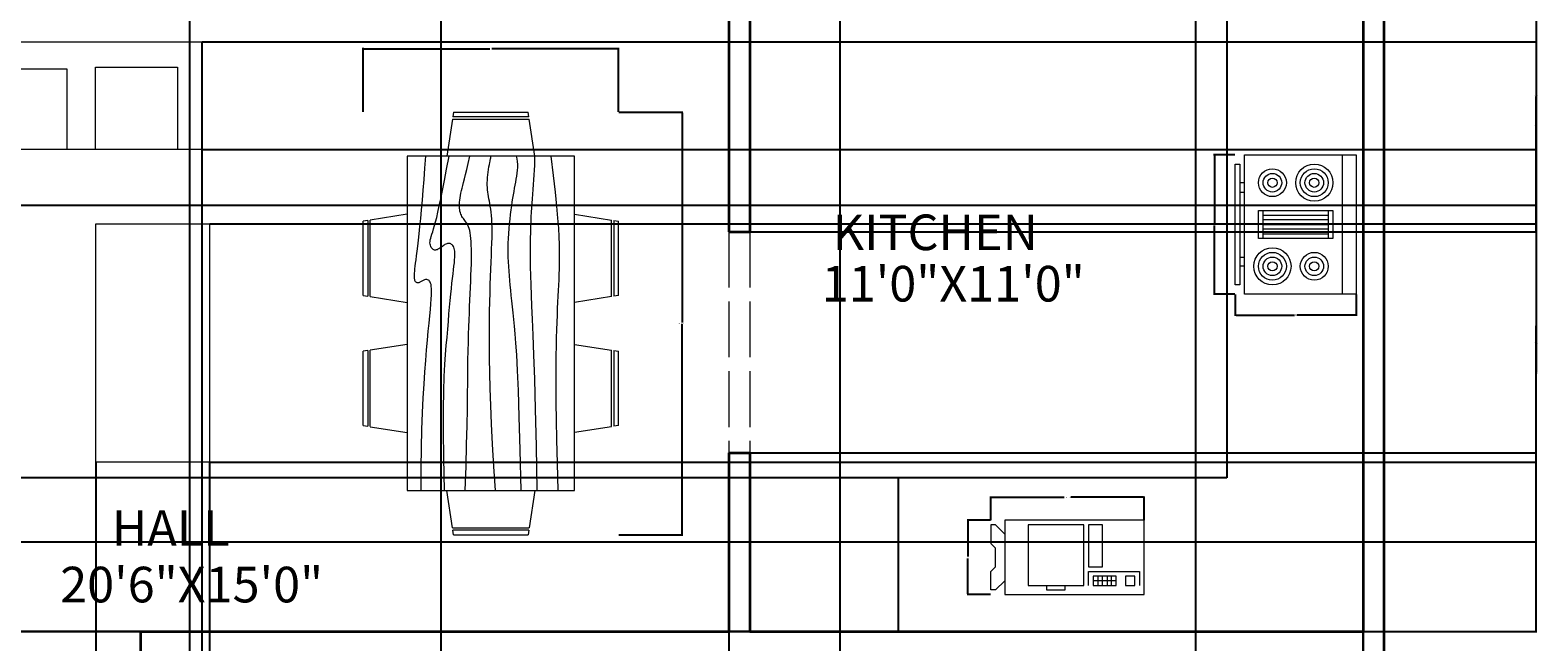
# Model space of a CAD drawing. Units: inches. Extents: x 2337 to 2851, y 1463 to 2183.
# Tile 3 of 4: x 2527 to 2851, y 1810 to 1942. Entities that reach past the tile are written whole.
import ezdxf

# ---------------------------------------------------------------- set-up
doc = ezdxf.new("R2010")
doc.units = ezdxf.units.IN
doc.linetypes.add('ACAD_ISO02W100', pattern=[15, 12, -3])
for name, color, linetype, lineweight in [('A-ANNO-DIMS', 2, 'Continuous', 18), ('A-AREA-IDEN', 7, 'Continuous', 18), ('A-EQPM', 9, 'Continuous', 18), ('A-FLOR-CASE', 8, 'Continuous', 25), ('A-FURN', 8, 'Continuous', 18), ('A-WALL', 7, 'Continuous', 35), ('A-WALL-OVHD', 7, 'ACAD_ISO02W100', 18)]:
    doc.layers.add(name, color=color, linetype=linetype, lineweight=lineweight)
doc.styles.get("Standard").update_dxf_attribs({"font": 'arial.ttf'})
doc.dimstyles.get("Standard").update_dxf_attribs({"dimtxt": 0.18, "dimasz": 0.18, "dimexe": 0.18, "dimexo": 0.0625, "dimgap": 0.09, "dimtad": 0, "dimtih": 1, "dimtoh": 1, "dimdec": 4, "dimzin": 0, "dimdsep": 46, "dimtxsty": 'Standard', "dimcen": 0.09, "dimadec": 0, "dimazin": 0, "dimtfac": 1, "dimtdec": 4, "dimtofl": 0, "dimtmove": 0, "dimatfit": 3, "dimfxl": 1, "dimtolj": 1, "dimtzin": 0, "dimarcsym": 0})

# ---------------------------------------------------------------- blocks, each defined once
blk = doc.blocks.new('Range-Oven - 30 in top')
for p, q in [((0, -3), (30, -3)), ((12, -6), (18, -6)), ((13, -20), (13, -6)), ((14, -6), (14, -20)), ((15, -20), (15, -6)), ((16, -6), (16, -20)), ((17, -20), (17, -6)), ((18, -20), (12, -20)), ((6, -24), (6, -25)), ((8, -25), (8, -24)), ((22, -25), (22, -24)), ((24, -24), (24, -25))]:
    blk.add_line(p, q)
for points in [[(0, -24), (0, 0), (30, 0), (30, -24)], [(12, -21), (12, -5), (18, -5), (18, -21)], [(2, -26), (2, -25), (28, -25), (28, -26)]]:
    blk.add_lwpolyline(points, close=True)
for centre, radius in [((6, -9), 4), ((6, -9), 3), ((24, -9), 3), ((6, -9), 2), ((6, -9), 1), ((24, -9), 2), ((24, -9), 1), ((6, -18), 3), ((6, -18), 2), ((24, -18), 4), ((24, -18), 3), ((24, -18), 2), ((6, -18), 1), ((24, -18), 1)]:
    blk.add_circle(centre, radius)
blk = doc.blocks.new('Copy Machine')
for p, q in [((0, 0), (0, -16)), ((30, 0), (0, 0)), ((30, -16), (30, 0)), ((-3, -1), (-3, -5)), ((-2, -1), (-3, -1)), ((0, -3), (-2, -1)), ((5, -1), (5, -14)), ((17, -1), (5, -1)), ((17, -14), (17, -1)), ((18, -1), (18, -10)), ((21, -1), (18, -1)), ((21, -10), (21, -1)), ((-3, -5), (-2, -6)), ((-2, -10), (-2, -6)), ((-3, -11), (-2, -10)), ((-3, -15), (-3, -11)), ((18, -10), (21, -10)), ((18, -14), (18, -11)), ((18, -11), (29, -11)), ((24, -12), (19, -12)), ((19, -12), (19, -14)), ((20, -12), (20, -14)), ((21, -14), (21, -12)), ((22, -12), (22, -14)), ((23, -14), (23, -12)), ((24, -14), (24, -12)), ((28, -12), (26, -12)), ((26, -12), (26, -14)), ((28, -14), (28, -12)), ((29, -11), (29, -14)), ((-2, -15), (-3, -15)), ((0, -13), (-2, -15)), ((0, -16), (30, -16)), ((5, -14), (17, -14)), ((9, -14), (9, -15)), ((9, -15), (13, -15)), ((13, -15), (13, -14)), ((24, -13), (19, -13)), ((19, -14), (24, -14)), ((26, -14), (28, -14))]:
    blk.add_line(p, q)
blk = doc.blocks.new('Dining Set - 36 x 72 in.')
for p, q in [((-22.2343, 26.00059), (-23.4847, 17.99762)), ((-22.2304, 26), (-5.7608, 26)), ((-22, 27.5), (-22.1562, 26.50042)), ((-5.8416, 26.5), (-22.1534, 26.5)), ((-22, 27.5), (-6, 27.5)), ((-5.8437, 26.49966), (-6, 27.5)), ((-4.5152, 17.99762), (-5.7655, 25.99926)), ((5.7657, 26.00059), (4.5153, 17.99762)), ((5.7696, 26), (22.2392, 26)), ((6, 27.5), (5.8438, 26.50042)), ((22.1584, 26.5), (5.8466, 26.5)), ((6, 27.5), (22, 27.5)), ((22.1563, 26.49966), (22, 27.5)), ((23.4848, 17.99762), (22.2345, 25.99926)), ((36, 18), (-36, 18)), ((-36, 18), (-36, -18)), ((36, -18), (36, 18)), ((-45.5, 8), (-44.5004, 8.15617)), ((-45.5, 8), (-45.5, -8)), ((-44.5, -8.15843), (-44.5, 8.15338)), ((-44.0006, 8.23428), (-35.9976, 9.48474)), ((-44, 8.23041), (-44, -8.23915)), ((44.0006, 8.23428), (35.9976, 9.48474)), ((44, 8.23041), (44, -8.23915)), ((44.5, -8.15843), (44.5, 8.15338)), ((45.5, 8), (44.5005, 8.15617)), ((45.5, 8), (45.5, -8)), ((-44.4997, -8.15631), (-45.5, -8)), ((-35.9976, -9.48476), (-43.9993, -8.2345)), ((35.9976, -9.48476), (43.9993, -8.2345)), ((44.4997, -8.15631), (45.5, -8)), ((-36, -18), (36, -18)), ((-22.2343, -26.0006), (-23.4847, -17.99762)), ((-4.5152, -17.99762), (-5.7655, -25.99928)), ((5.7657, -26.0006), (4.5153, -17.99762)), ((23.4848, -17.99762), (22.2345, -25.99928)), ((-22.2304, -26), (-5.7608, -26)), ((-22, -27.5), (-22.1562, -26.50044)), ((-5.8416, -26.5), (-22.1534, -26.5)), ((-22, -27.5), (-6, -27.5)), ((-5.8437, -26.49967), (-6, -27.5)), ((5.7696, -26), (22.2392, -26)), ((6, -27.5), (5.8438, -26.50044)), ((22.1584, -26.5), (5.8466, -26.5)), ((6, -27.5), (22, -27.5)), ((22.1563, -26.49967), (22, -27.5))]:
    blk.add_line(p, q)
for points in [[(-36, 15), (-31.1772, 14.97754), (-26.8079, 14.91406), (-22.8538, 14.81543), (-19.276, 14.6875), (-16.0362, 14.53613), (-13.0957, 14.36718), (-10.4159, 14.18652), (-7.9583, 14), (-5.6904, 13.81315), (-3.6035, 13.63021), (-1.6954, 13.45508), (0.0365, 13.29166), (1.5945, 13.14388), (2.9811, 13.01562), (4.1988, 12.9108), (5.25, 12.83333), (6.1393, 12.78613), (6.8802, 12.76823), (7.4883, 12.77767), (7.9792, 12.8125), (8.3685, 12.87077), (8.6719, 12.95052), (8.9049, 13.0498), (9.0833, 13.16666), (9.2205, 13.29899), (9.3216, 13.44401), (9.3895, 13.59879), (9.4271, 13.76041), (9.4373, 13.92594), (9.4232, 14.09245), (9.3875, 14.257), (9.3333, 14.41666), (9.2638, 14.56917), (9.1836, 14.71484), (9.0975, 14.85465), (9.0104, 14.98958), (8.9272, 15.1206), (8.8529, 15.2487), (8.7922, 15.37483), (8.75, 15.5), (8.7305, 15.62467), (8.7344, 15.74739), (8.7617, 15.86621), (8.8125, 15.97916), (8.8867, 16.08431), (8.9844, 16.17968), (9.1055, 16.26334), (9.25, 16.33333), (9.4189, 16.38802), (9.6172, 16.42708), (9.8506, 16.45052), (10.125, 16.45833), (10.4463, 16.45052), (10.8203, 16.42708), (11.2529, 16.38802), (11.75, 16.33333), (12.3184, 16.26318), (12.9694, 16.17838), (13.7151, 16.07991), (14.5677, 15.96875), (15.5395, 15.84586), (16.6426, 15.71224), (17.8893, 15.56884), (19.2917, 15.41666), (20.859, 15.25667), (22.5879, 15.08984), (24.4721, 14.91715), (26.5052, 14.73958), (28.6809, 14.5581), (30.9929, 14.3737), (33.4347, 14.18733), (36, 14)], [(-36, 10), (-28.9766, 10.14274), (-23.1725, 10.20442), (-18.4241, 10.19775), (-14.5677, 10.13541), (-11.4399, 10.03011), (-8.877, 9.89453), (-6.7154, 9.74137), (-4.7917, 9.58333), (-2.9698, 9.43082), (-1.2246, 9.28515), (0.4415, 9.14534), (2.026, 9.01041), (3.5266, 8.87939), (4.9408, 8.7513), (6.266, 8.62516), (7.5, 8.5), (8.6411, 8.37549), (9.6914, 8.2539), (10.6538, 8.13818), (11.5312, 8.03125), (12.3267, 7.93603), (13.043, 7.85547), (13.6831, 7.79248), (14.25, 7.75), (14.7471, 7.7303), (15.1797, 7.73307), (15.5537, 7.75732), (15.875, 7.80208), (16.1494, 7.86637), (16.3828, 7.94922), (16.5811, 8.04964), (16.75, 8.16666), (16.8944, 8.29915), (17.0143, 8.44531), (17.1089, 8.60319), (17.1771, 8.77083), (17.218, 8.94629), (17.2305, 9.1276), (17.2137, 9.31282), (17.1667, 9.5), (17.0895, 9.6875), (16.987, 9.875), (16.8649, 10.0625), (16.7292, 10.25), (16.5856, 10.4375), (16.4401, 10.625), (16.2985, 10.8125), (16.1667, 11), (16.05, 11.18733), (15.9518, 11.3737), (15.8752, 11.5581), (15.8229, 11.73958), (15.798, 11.91715), (15.8034, 12.08984), (15.842, 12.25667), (15.9167, 12.41666), (16.0295, 12.56836), (16.1784, 12.70833), (16.3605, 12.83268), (16.5729, 12.9375), (16.8127, 13.01888), (17.0768, 13.07291), (17.3625, 13.0957), (17.6667, 13.08333), (17.9894, 13.03312), (18.3418, 12.94726), (18.7382, 12.82918), (19.1927, 12.68229), (19.7195, 12.51001), (20.3327, 12.31575), (21.0465, 12.10294), (21.875, 11.875), (22.8357, 11.63354), (23.959, 11.37304), (25.2786, 11.08618), (26.8282, 10.76562), (28.6414, 10.40405), (30.752, 9.99414), (33.1936, 9.52856), (36, 9)], [(-36, 5.5), (-30.7157, 5.3348), (-26.069, 5.20963), (-21.9946, 5.11767), (-18.4271, 5.05208), (-15.3009, 5.00602), (-12.5508, 4.97265), (-10.1112, 4.94515), (-7.9167, 4.91666), (-5.909, 4.88167), (-4.0586, 4.83984), (-2.3429, 4.79215), (-0.7396, 4.73958), (0.7739, 4.6831), (2.22, 4.6237), (3.6213, 4.56233), (5, 4.5), (6.373, 4.43782), (7.7344, 4.3776), (9.0723, 4.32129), (10.375, 4.27083), (11.6309, 4.22819), (12.8281, 4.19531), (13.9551, 4.17415), (15, 4.16666), (15.954, 4.17448), (16.819, 4.19791), (17.6001, 4.23698), (18.3021, 4.29166), (18.9299, 4.36198), (19.4883, 4.44791), (19.9823, 4.54948), (20.4167, 4.66666), (20.7969, 4.79899), (21.1302, 4.94401), (21.4245, 5.09879), (21.6875, 5.26041), (21.9271, 5.42594), (22.1511, 5.59245), (22.3672, 5.757), (22.5834, 5.91666), (22.8065, 6.06868), (23.0404, 6.21093), (23.2879, 6.34147), (23.5521, 6.45833), (23.8358, 6.55957), (24.142, 6.64323), (24.4735, 6.70735), (24.8334, 6.75), (25.2235, 6.76969), (25.642, 6.76692), (26.0858, 6.74267), (26.5521, 6.69791), (27.0379, 6.63362), (27.5404, 6.55078), (28.0565, 6.45036), (28.5834, 6.33333), (29.1242, 6.19987), (29.7071, 6.04687), (30.3661, 5.87044), (31.1354, 5.66666), (32.0493, 5.43164), (33.142, 5.16146), (34.4475, 4.85221), (36, 4.5)], [(-36, -1), (-30.7915, -0.6591), (-26.0195, -0.38216), (-21.6519, -0.16284), (-17.6563, 0.00521), (-14.0005, 0.12833), (-10.6523, 0.21289), (-7.5796, 0.26522), (-4.75, 0.29166), (-2.134, 0.29793), (0.2878, 0.28711), (2.5317, 0.26163), (4.6146, 0.22396), (6.5529, 0.17651), (8.3633, 0.12174), (10.0623, 0.06209), (11.6667, 0), (13.1899, -0.06201), (14.6341, -0.1211), (15.9982, -0.17432), (17.2813, -0.21875), (18.4823, -0.25147), (19.6003, -0.26953), (20.6343, -0.27002), (21.5834, -0.25), (22.4481, -0.20768), (23.2357, -0.14584), (23.9549, -0.06836), (24.6146, 0.02083), (25.2235, 0.11784), (25.7904, 0.21875), (26.3241, 0.31966), (26.8334, 0.41666), (27.3265, 0.50618), (27.8099, 0.58593), (28.2894, 0.65397), (28.7709, 0.70833), (29.2601, 0.74707), (29.763, 0.76823), (30.2855, 0.76985), (30.8334, 0.75), (31.4088, 0.70784), (31.9994, 0.64713), (32.589, 0.57275), (33.1615, 0.48958), (33.7008, 0.4025), (34.1908, 0.3164), (34.6153, 0.23616), (34.9584, 0.16666), (35.2099, 0.11165), (35.3848, 0.07031), (35.504, 0.04069), (35.5886, 0.02083), (35.6594, 0.00879), (35.7377, 0.0026), (35.8442, 0.00032), (36, 0)], [(-36, -6.5), (-27.1843, -6.31267), (-20.084, -6.1263), (-14.469, -5.9419), (-10.1094, -5.76042), (-6.7752, -5.58285), (-4.2363, -5.41016), (-2.2629, -5.24333), (-0.625, -5.08334), (0.8708, -4.93099), (2.2715, -4.78646), (3.5872, -4.64974), (4.8281, -4.52084), (6.0046, -4.39974), (7.127, -4.28646), (8.2053, -4.18099), (9.25, -4.08334), (10.2705, -3.99382), (11.2734, -3.91407), (12.2647, -3.84603), (13.25, -3.79167), (14.2354, -3.75293), (15.2266, -3.73177), (16.2295, -3.73015), (17.25, -3.75), (18.2912, -3.79248), (19.3451, -3.85547), (20.4009, -3.93604), (21.4479, -4.03125), (22.4754, -4.13819), (23.4727, -4.25391), (24.4289, -4.37549), (25.3334, -4.5), (26.1785, -4.62492), (26.9694, -4.74935), (27.7145, -4.87281), (28.4219, -4.99479), (29.1, -5.11483), (29.7572, -5.23242), (30.4016, -5.34709), (31.0417, -5.45834), (31.6837, -5.56437), (32.3262, -5.65821), (32.9658, -5.73153), (33.599, -5.77604), (34.2224, -5.78345), (34.8327, -5.74545), (35.4264, -5.65373), (36, -5.5)], [(-36, -10), (-26.4022, -9.81299), (-18.4675, -9.62891), (-11.9839, -9.45069), (-6.7396, -9.28125), (-2.5226, -9.12354), (0.8789, -8.98047), (3.6769, -8.85498), (6.0833, -8.75), (8.2767, -8.66765), (10.3021, -8.60677), (12.1712, -8.56543), (13.8958, -8.54167), (15.4876, -8.53353), (16.9583, -8.53907), (18.3197, -8.55632), (19.5834, -8.58334), (20.7616, -8.61841), (21.8685, -8.66081), (22.9188, -8.71004), (23.9271, -8.76563), (24.9081, -8.82707), (25.8763, -8.89388), (26.8465, -8.96558), (27.8334, -9.04167), (28.8474, -9.12118), (29.8828, -9.20117), (30.93, -9.27824), (31.9792, -9.34896), (33.0205, -9.40991), (34.0443, -9.45768), (35.0407, -9.48885), (36, -9.5)], [(-36, -14.5), (-30.0881, -14.33513), (-25.0332, -14.21224), (-20.7312, -14.12647), (-17.0781, -14.07292), (-13.97, -14.04671), (-11.3027, -14.04297), (-8.9724, -14.05681), (-6.875, -14.08334), (-4.9224, -14.11833), (-3.0905, -14.16016), (-1.3709, -14.20785), (0.2448, -14.26042), (1.7647, -14.3169), (3.1973, -14.3763), (4.5507, -14.43767), (5.8333, -14.5), (7.0554, -14.5621), (8.235, -14.62175), (9.3922, -14.67652), (10.5469, -14.72396), (11.7192, -14.76164), (12.929, -14.78711), (14.1965, -14.79794), (15.5417, -14.79167), (16.9933, -14.76424), (18.6152, -14.70508), (20.4804, -14.60197), (22.6615, -14.44271), (25.2312, -14.21509), (28.2624, -13.9069), (31.8277, -13.50594), (36, -13)]]:
    blk.add_lwpolyline(points)
blk = doc.blocks.new('*D23')
at = {"layer": 'A-ANNO-DIMS', "color": 0, "lineweight": -2, "transparency": 16777216}
for p, q in [((2785.97, 1914.93), (2781.36, 1914.93)), ((2781.54, 1914.75), (2781.54, 1900.11)), ((2781.54, 1885.11), (2781.54, 1899.75)), ((2785.97, 1884.93), (2781.36, 1884.93))]:
    blk.add_line(p, q, dxfattribs=at)
at = {"layer": 'A-ANNO-DIMS', "color": 0, "transparency": 16777216}
for points in [[(2781.51, 1914.75), (2781.57, 1914.75), (2781.54, 1914.93)], [(2781.51, 1885.11), (2781.57, 1885.11), (2781.54, 1884.93)]]:
    blk.add_solid(points, dxfattribs=at)
at = {"layer": 'Defpoints', "color": 0, "transparency": 16777216}
for p in [(2786.04, 1914.93), (2781.54, 1884.93), (2786.04, 1884.93)]:
    blk.add_point(p, dxfattribs=at)
at = {"layer": 'A-ANNO-DIMS', "color": 0, "transparency": 16777216, "insert": (2781.54, 1899.93), "char_height": 0.18, "attachment_point": 5}
blk.add_mtext('\\A1;RANGE 30', dxfattribs=at)
blk = doc.blocks.new('*D24')
at = {"layer": 'A-ANNO-DIMS', "color": 0, "lineweight": -2, "transparency": 16777216}
for p, q in [((2786.04, 1884.87), (2786.04, 1880.25)), ((2812.04, 1884.87), (2812.04, 1880.25)), ((2786.22, 1880.43), (2798.81, 1880.43)), ((2811.86, 1880.43), (2799.26, 1880.43))]:
    blk.add_line(p, q, dxfattribs=at)
at = {"layer": 'A-ANNO-DIMS', "color": 0, "transparency": 16777216}
for points in [[(2786.22, 1880.46), (2786.22, 1880.4), (2786.04, 1880.43)], [(2811.86, 1880.46), (2811.86, 1880.4), (2812.04, 1880.43)]]:
    blk.add_solid(points, dxfattribs=at)
at = {"layer": 'Defpoints', "color": 0, "transparency": 16777216}
for p in [(2786.04, 1884.93), (2812.04, 1884.93), (2812.04, 1880.43)]:
    blk.add_point(p, dxfattribs=at)
at = {"layer": 'A-ANNO-DIMS', "color": 0, "transparency": 16777216, "insert": (2799.04, 1880.43), "char_height": 0.18, "attachment_point": 5}
blk.add_mtext('\\A1;26', dxfattribs=at)
blk = doc.blocks.new('*D25')
at = {"layer": 'A-ANNO-DIMS', "color": 0, "lineweight": -2, "transparency": 16777216}
for p, q in [((2733.44, 1836.31), (2733.44, 1841.38)), ((2733.62, 1841.2), (2749.2, 1841.2)), ((2766.26, 1841.2), (2750.67, 1841.2)), ((2766.44, 1836.31), (2766.44, 1841.38))]:
    blk.add_line(p, q, dxfattribs=at)
at = {"layer": 'A-ANNO-DIMS', "color": 0, "transparency": 16777216}
for points in [[(2733.62, 1841.23), (2733.62, 1841.17), (2733.44, 1841.2)], [(2766.26, 1841.23), (2766.26, 1841.17), (2766.44, 1841.2)]]:
    blk.add_solid(points, dxfattribs=at)
at = {"layer": 'Defpoints', "color": 0, "transparency": 16777216}
for p in [(2766.44, 1841.2), (2733.44, 1836.25), (2766.44, 1836.25)]:
    blk.add_point(p, dxfattribs=at)
at = {"layer": 'A-ANNO-DIMS', "color": 0, "transparency": 16777216, "insert": (2749.94, 1841.2), "char_height": 0.18, "attachment_point": 5}
blk.add_mtext('\\A1;COPIER 33', dxfattribs=at)
blk = doc.blocks.new('*D26')
at = {"layer": 'A-ANNO-DIMS', "color": 0, "lineweight": -2, "transparency": 16777216}
for p, q in [((2733.37, 1836.25), (2728.31, 1836.25)), ((2728.49, 1836.07), (2728.49, 1828.43)), ((2728.49, 1820.43), (2728.49, 1828.06)), ((2733.37, 1820.25), (2728.31, 1820.25))]:
    blk.add_line(p, q, dxfattribs=at)
at = {"layer": 'A-ANNO-DIMS', "color": 0, "transparency": 16777216}
for points in [[(2728.46, 1836.07), (2728.52, 1836.07), (2728.49, 1836.25)], [(2728.46, 1820.43), (2728.52, 1820.43), (2728.49, 1820.25)]]:
    blk.add_solid(points, dxfattribs=at)
at = {"layer": 'Defpoints', "color": 0, "transparency": 16777216}
for p in [(2728.49, 1836.25), (2733.44, 1836.25), (2733.44, 1820.25)]:
    blk.add_point(p, dxfattribs=at)
at = {"layer": 'A-ANNO-DIMS', "color": 0, "transparency": 16777216, "insert": (2728.49, 1828.25), "char_height": 0.18, "attachment_point": 5}
blk.add_mtext('\\A1;16', dxfattribs=at)
blk = doc.blocks.new('*D27')
at = {"layer": 'A-ANNO-DIMS', "color": 0, "lineweight": -2, "transparency": 16777216}
for p, q in [((2653.4, 1924.14), (2667.16, 1924.14)), ((2666.98, 1923.96), (2666.98, 1878.82)), ((2666.98, 1833.32), (2666.98, 1878.46)), ((2653.4, 1833.14), (2667.16, 1833.14))]:
    blk.add_line(p, q, dxfattribs=at)
at = {"layer": 'A-ANNO-DIMS', "color": 0, "transparency": 16777216}
for points in [[(2666.95, 1923.96), (2667.01, 1923.96), (2666.98, 1924.14)], [(2666.95, 1833.32), (2667.01, 1833.32), (2666.98, 1833.14)]]:
    blk.add_solid(points, dxfattribs=at)
at = {"layer": 'Defpoints', "color": 0, "transparency": 16777216}
for p in [(2653.33, 1924.14), (2666.98, 1924.14), (2653.33, 1833.14)]:
    blk.add_point(p, dxfattribs=at)
at = {"layer": 'A-ANNO-DIMS', "color": 0, "transparency": 16777216, "insert": (2666.98, 1878.64), "char_height": 0.18, "attachment_point": 5}
blk.add_mtext('\\A1;DINING SET 91', dxfattribs=at)
blk = doc.blocks.new('*D28')
at = {"layer": 'A-ANNO-DIMS', "color": 0, "lineweight": -2, "transparency": 16777216}
for p, q in [((2598.33, 1924.2), (2598.33, 1937.97)), ((2598.51, 1937.79), (2625.61, 1937.79)), ((2653.15, 1937.79), (2626.05, 1937.79)), ((2653.33, 1924.2), (2653.33, 1937.97))]:
    blk.add_line(p, q, dxfattribs=at)
at = {"layer": 'A-ANNO-DIMS', "color": 0, "transparency": 16777216}
for points in [[(2598.51, 1937.82), (2598.51, 1937.76), (2598.33, 1937.79)], [(2653.15, 1937.82), (2653.15, 1937.76), (2653.33, 1937.79)]]:
    blk.add_solid(points, dxfattribs=at)
at = {"layer": 'Defpoints', "color": 0, "transparency": 16777216}
for p in [(2598.33, 1937.79), (2598.33, 1924.14), (2653.33, 1924.14)]:
    blk.add_point(p, dxfattribs=at)
at = {"layer": 'A-ANNO-DIMS', "color": 0, "transparency": 16777216, "insert": (2625.83, 1937.79), "char_height": 0.18, "attachment_point": 5}
blk.add_mtext('\\A1;55', dxfattribs=at)
blk = doc.blocks.new('*D32')
at = {"layer": 'A-ANNO-DIMS', "color": 0, "lineweight": -2, "transparency": 16777216}
for p, q in [((2561.04, 1627.89), (2561.04, 2182.75)), ((2561.22, 2182.57), (2630.76, 2182.57)), ((2700.86, 2182.57), (2631.32, 2182.57)), ((2701.04, 1627.89), (2701.04, 2182.75))]:
    blk.add_line(p, q, dxfattribs=at)
at = {"layer": 'A-ANNO-DIMS', "color": 0, "transparency": 16777216}
for points in [[(2561.22, 2182.6), (2561.22, 2182.54), (2561.04, 2182.57)], [(2700.86, 2182.6), (2700.86, 2182.54), (2701.04, 2182.57)]]:
    blk.add_solid(points, dxfattribs=at)
at = {"layer": 'Defpoints', "color": 0, "transparency": 16777216}
for p in [(2701.04, 2182.57), (2561.04, 1627.83), (2701.04, 1627.83)]:
    blk.add_point(p, dxfattribs=at)
at = {"layer": 'A-ANNO-DIMS', "color": 0, "transparency": 16777216, "insert": (2631.04, 2182.57), "char_height": 0.18, "attachment_point": 5}
blk.add_mtext('\\A1;140', dxfattribs=at)
blk = doc.blocks.new('*D35')
at = {"layer": 'A-ANNO-DIMS', "color": 0, "lineweight": -2, "transparency": 16777216}
for p, q in [((2489.04, 1812.27), (2489.04, 1462.52)), ((2677.04, 1812.27), (2677.04, 1462.52)), ((2489.22, 1462.7), (2582.76, 1462.7)), ((2676.86, 1462.7), (2583.32, 1462.7))]:
    blk.add_line(p, q, dxfattribs=at)
at = {"layer": 'A-ANNO-DIMS', "color": 0, "transparency": 16777216}
for points in [[(2489.22, 1462.73), (2489.22, 1462.67), (2489.04, 1462.7)], [(2676.86, 1462.73), (2676.86, 1462.67), (2677.04, 1462.7)]]:
    blk.add_solid(points, dxfattribs=at)
at = {"layer": 'Defpoints', "color": 0, "transparency": 16777216}
for p in [(2489.04, 1812.33), (2677.04, 1812.33), (2677.04, 1462.7)]:
    blk.add_point(p, dxfattribs=at)
at = {"layer": 'A-ANNO-DIMS', "color": 0, "transparency": 16777216, "insert": (2583.04, 1462.7), "char_height": 0.18, "attachment_point": 5}
blk.add_mtext('\\A1;188', dxfattribs=at)
blk = doc.blocks.new('*D36')
at = {"layer": 'A-ANNO-DIMS', "color": 0, "lineweight": -2, "transparency": 16777216}
for p, q in [((2489.1, 1944.33), (2850.96, 1944.33)), ((2850.78, 1944.15), (2850.78, 1878.51)), ((2850.78, 1812.51), (2850.78, 1878.15)), ((2489.1, 1812.33), (2850.96, 1812.33))]:
    blk.add_line(p, q, dxfattribs=at)
at = {"layer": 'A-ANNO-DIMS', "color": 0, "transparency": 16777216}
for points in [[(2850.75, 1944.15), (2850.81, 1944.15), (2850.78, 1944.33)], [(2850.75, 1812.51), (2850.81, 1812.51), (2850.78, 1812.33)]]:
    blk.add_solid(points, dxfattribs=at)
at = {"layer": 'Defpoints', "color": 0, "transparency": 16777216}
for p in [(2489.04, 1944.33), (2850.78, 1944.33), (2489.04, 1812.33)]:
    blk.add_point(p, dxfattribs=at)
at = {"layer": 'A-ANNO-DIMS', "color": 0, "transparency": 16777216, "insert": (2850.78, 1878.33), "char_height": 0.18, "attachment_point": 5}
blk.add_mtext('\\A1;132', dxfattribs=at)
blk = doc.blocks.new('*D37')
at = {"layer": 'A-ANNO-DIMS', "color": 0, "lineweight": -2, "transparency": 16777216}
for p, q in [((2615.04, 2080.77), (2615.04, 1462.52)), ((2813.54, 2080.77), (2813.54, 1462.52)), ((2615.22, 1462.7), (2713.9, 1462.7)), ((2813.36, 1462.7), (2714.67, 1462.7))]:
    blk.add_line(p, q, dxfattribs=at)
at = {"layer": 'A-ANNO-DIMS', "color": 0, "transparency": 16777216}
for points in [[(2615.22, 1462.73), (2615.22, 1462.67), (2615.04, 1462.7)], [(2813.36, 1462.73), (2813.36, 1462.67), (2813.54, 1462.7)]]:
    blk.add_solid(points, dxfattribs=at)
at = {"layer": 'Defpoints', "color": 0, "transparency": 16777216}
for p in [(2615.04, 2080.83), (2813.54, 2080.83), (2813.54, 1462.7)]:
    blk.add_point(p, dxfattribs=at)
at = {"layer": 'A-ANNO-DIMS', "color": 0, "transparency": 16777216, "insert": (2714.29, 1462.7), "char_height": 0.18, "attachment_point": 5}
blk.add_mtext('\\A1;198.5', dxfattribs=at)
blk = doc.blocks.new('*D41')
at = {"layer": 'A-ANNO-DIMS', "color": 0, "lineweight": -2, "transparency": 16777216}
for p, q in [((2681.6, 1898.34), (2850.96, 1898.34)), ((2850.78, 1898.16), (2850.78, 1874.75)), ((2850.78, 1850.99), (2850.78, 1874.39)), ((2681.6, 1850.81), (2850.96, 1850.81))]:
    blk.add_line(p, q, dxfattribs=at)
at = {"layer": 'A-ANNO-DIMS', "color": 0, "transparency": 16777216}
for points in [[(2850.75, 1898.16), (2850.81, 1898.16), (2850.78, 1898.34)], [(2850.75, 1850.99), (2850.81, 1850.99), (2850.78, 1850.81)]]:
    blk.add_solid(points, dxfattribs=at)
at = {"layer": 'Defpoints', "color": 0, "transparency": 16777216}
for p in [(2681.54, 1898.34), (2850.78, 1898.34), (2681.54, 1850.81)]:
    blk.add_point(p, dxfattribs=at)
at = {"layer": 'A-ANNO-DIMS', "color": 0, "transparency": 16777216, "insert": (2850.78, 1874.57), "char_height": 0.18, "attachment_point": 5}
blk.add_mtext('\\A1;47.53', dxfattribs=at)
blk = doc.blocks.new('*D42')
at = {"layer": 'A-ANNO-DIMS', "color": 0, "lineweight": -2, "transparency": 16777216}
for p, q in [((2681.6, 1944.33), (2850.96, 1944.33)), ((2850.78, 1944.15), (2850.78, 1921.51)), ((2850.78, 1898.52), (2850.78, 1921.15)), ((2681.6, 1898.34), (2850.96, 1898.34))]:
    blk.add_line(p, q, dxfattribs=at)
at = {"layer": 'A-ANNO-DIMS', "color": 0, "transparency": 16777216}
for points in [[(2850.75, 1944.15), (2850.81, 1944.15), (2850.78, 1944.33)], [(2850.75, 1898.52), (2850.81, 1898.52), (2850.78, 1898.34)]]:
    blk.add_solid(points, dxfattribs=at)
at = {"layer": 'Defpoints', "color": 0, "transparency": 16777216}
for p in [(2681.54, 1944.33), (2850.78, 1944.33), (2681.54, 1898.34)]:
    blk.add_point(p, dxfattribs=at)
at = {"layer": 'A-ANNO-DIMS', "color": 0, "transparency": 16777216, "insert": (2850.78, 1921.33), "char_height": 0.18, "attachment_point": 5}
blk.add_mtext('\\A1;45.99', dxfattribs=at)
blk = doc.blocks.new('*D45')
at = {"layer": 'A-ANNO-DIMS', "color": 0, "lineweight": -2, "transparency": 16777216}
for p, q in [((2777.54, 1699.89), (2777.54, 2182.75)), ((2777.72, 2182.57), (2795.32, 2182.57)), ((2813.36, 2182.57), (2795.76, 2182.57)), ((2813.54, 1699.89), (2813.54, 2182.75))]:
    blk.add_line(p, q, dxfattribs=at)
at = {"layer": 'A-ANNO-DIMS', "color": 0, "transparency": 16777216}
for points in [[(2777.72, 2182.6), (2777.72, 2182.54), (2777.54, 2182.57)], [(2813.36, 2182.6), (2813.36, 2182.54), (2813.54, 2182.57)]]:
    blk.add_solid(points, dxfattribs=at)
at = {"layer": 'Defpoints', "color": 0, "transparency": 16777216}
for p in [(2813.54, 2182.57), (2777.54, 1699.83), (2813.54, 1699.83)]:
    blk.add_point(p, dxfattribs=at)
at = {"layer": 'A-ANNO-DIMS', "color": 0, "transparency": 16777216, "insert": (2795.54, 2182.57), "char_height": 0.18, "attachment_point": 5}
blk.add_mtext('\\A1;36', dxfattribs=at)
blk = doc.blocks.new('*D48')
at = {"layer": 'A-ANNO-DIMS', "color": 0, "lineweight": -2, "transparency": 16777216}
for p, q in [((2713.4, 1845.41), (2336.95, 1845.41)), ((2337.13, 1845.23), (2337.13, 1829.05)), ((2337.13, 1812.51), (2337.13, 1828.69)), ((2713.4, 1812.33), (2336.95, 1812.33))]:
    blk.add_line(p, q, dxfattribs=at)
at = {"layer": 'A-ANNO-DIMS', "color": 0, "transparency": 16777216}
for points in [[(2337.1, 1845.23), (2337.16, 1845.23), (2337.13, 1845.41)], [(2337.1, 1812.51), (2337.16, 1812.51), (2337.13, 1812.33)]]:
    blk.add_solid(points, dxfattribs=at)
at = {"layer": 'Defpoints', "color": 0, "transparency": 16777216}
for p in [(2337.13, 1845.41), (2713.47, 1845.41), (2713.47, 1812.33)]:
    blk.add_point(p, dxfattribs=at)
at = {"layer": 'A-ANNO-DIMS', "color": 0, "transparency": 16777216, "insert": (2337.13, 1828.87), "char_height": 0.18, "attachment_point": 5}
blk.add_mtext('\\A1;33.08', dxfattribs=at)
blk = doc.blocks.new('*D49')
at = {"layer": 'A-ANNO-DIMS', "color": 0, "lineweight": -2, "transparency": 16777216}
for p, q in [((2521.69, 1904.09), (2850.96, 1904.09)), ((2850.78, 1903.91), (2850.78, 1868.04)), ((2850.78, 1831.81), (2850.78, 1867.68)), ((2521.69, 1831.63), (2850.96, 1831.63))]:
    blk.add_line(p, q, dxfattribs=at)
at = {"layer": 'A-ANNO-DIMS', "color": 0, "transparency": 16777216}
for points in [[(2850.75, 1903.91), (2850.81, 1903.91), (2850.78, 1904.09)], [(2850.75, 1831.81), (2850.81, 1831.81), (2850.78, 1831.63)]]:
    blk.add_solid(points, dxfattribs=at)
at = {"layer": 'Defpoints', "color": 0, "transparency": 16777216}
for p in [(2521.63, 1904.09), (2850.78, 1904.09), (2521.63, 1831.63)]:
    blk.add_point(p, dxfattribs=at)
at = {"layer": 'A-ANNO-DIMS', "color": 0, "transparency": 16777216, "insert": (2850.78, 1867.86), "char_height": 0.18, "attachment_point": 5}
blk.add_mtext('\\A1;72.46', dxfattribs=at)
blk = doc.blocks.new('*D51')
at = {"layer": 'A-ANNO-DIMS', "color": 0, "lineweight": -2, "transparency": 16777216}
for p, q in [((2511.27, 1939.17), (2511.27, 1462.52)), ((2563.65, 1939.17), (2563.65, 1462.52)), ((2511.45, 1462.7), (2537.06, 1462.7)), ((2563.47, 1462.7), (2537.85, 1462.7))]:
    blk.add_line(p, q, dxfattribs=at)
at = {"layer": 'A-ANNO-DIMS', "color": 0, "transparency": 16777216}
for points in [[(2511.45, 1462.73), (2511.45, 1462.67), (2511.27, 1462.7)], [(2563.47, 1462.73), (2563.47, 1462.67), (2563.65, 1462.7)]]:
    blk.add_solid(points, dxfattribs=at)
at = {"layer": 'Defpoints', "color": 0, "transparency": 16777216}
for p in [(2511.27, 1939.23), (2563.65, 1939.23), (2563.65, 1462.7)]:
    blk.add_point(p, dxfattribs=at)
at = {"layer": 'A-ANNO-DIMS', "color": 0, "transparency": 16777216, "insert": (2537.46, 1462.7), "char_height": 0.18, "attachment_point": 5}
blk.add_mtext('\\A1;52.38', dxfattribs=at)
blk = doc.blocks.new('*D52')
at = {"layer": 'A-ANNO-DIMS', "color": 0, "lineweight": -2, "transparency": 16777216}
for p, q in [((2563.71, 1939.23), (2850.96, 1939.23)), ((2850.78, 1939.05), (2850.78, 1927.85)), ((2850.78, 1916.28), (2850.78, 1927.48)), ((2563.71, 1916.1), (2850.96, 1916.1))]:
    blk.add_line(p, q, dxfattribs=at)
at = {"layer": 'A-ANNO-DIMS', "color": 0, "transparency": 16777216}
for points in [[(2850.75, 1939.05), (2850.81, 1939.05), (2850.78, 1939.23)], [(2850.75, 1916.28), (2850.81, 1916.28), (2850.78, 1916.1)]]:
    blk.add_solid(points, dxfattribs=at)
at = {"layer": 'Defpoints', "color": 0, "transparency": 16777216}
for p in [(2563.65, 1939.23), (2850.78, 1939.23), (2563.65, 1916.1)]:
    blk.add_point(p, dxfattribs=at)
at = {"layer": 'A-ANNO-DIMS', "color": 0, "transparency": 16777216, "insert": (2850.78, 1927.67), "char_height": 0.18, "attachment_point": 5}
blk.add_mtext('\\A1;23.127', dxfattribs=at)
blk = doc.blocks.new('*D53')
at = {"layer": 'A-ANNO-DIMS', "color": 0, "lineweight": -2, "transparency": 16777216}
for p, q in [((2540.84, 1848.69), (2540.84, 1462.52)), ((2565.31, 1848.69), (2565.31, 1462.52)), ((2541.02, 1462.7), (2552.61, 1462.7)), ((2565.13, 1462.7), (2553.54, 1462.7))]:
    blk.add_line(p, q, dxfattribs=at)
at = {"layer": 'A-ANNO-DIMS', "color": 0, "transparency": 16777216}
for points in [[(2541.02, 1462.73), (2541.02, 1462.67), (2540.84, 1462.7)], [(2565.13, 1462.73), (2565.13, 1462.67), (2565.31, 1462.7)]]:
    blk.add_solid(points, dxfattribs=at)
at = {"layer": 'Defpoints', "color": 0, "transparency": 16777216}
for p in [(2540.84, 1848.75), (2565.31, 1848.75), (2565.31, 1462.7)]:
    blk.add_point(p, dxfattribs=at)
at = {"layer": 'A-ANNO-DIMS', "color": 0, "transparency": 16777216, "insert": (2553.08, 1462.7), "char_height": 0.18, "attachment_point": 5}
blk.add_mtext('\\A1;24.466', dxfattribs=at)
blk = doc.blocks.new('*D54')
at = {"layer": 'A-ANNO-DIMS', "color": 0, "lineweight": -2, "transparency": 16777216}
for p, q in [((2565.37, 1900.1), (2850.96, 1900.1)), ((2850.78, 1899.92), (2850.78, 1874.61)), ((2850.78, 1848.93), (2850.78, 1874.24)), ((2565.37, 1848.75), (2850.96, 1848.75))]:
    blk.add_line(p, q, dxfattribs=at)
at = {"layer": 'A-ANNO-DIMS', "color": 0, "transparency": 16777216}
for points in [[(2850.75, 1899.92), (2850.81, 1899.92), (2850.78, 1900.1)], [(2850.75, 1848.93), (2850.81, 1848.93), (2850.78, 1848.75)]]:
    blk.add_solid(points, dxfattribs=at)
at = {"layer": 'Defpoints', "color": 0, "transparency": 16777216}
for p in [(2565.31, 1900.1), (2850.78, 1900.1), (2565.31, 1848.75)]:
    blk.add_point(p, dxfattribs=at)
at = {"layer": 'A-ANNO-DIMS', "color": 0, "transparency": 16777216, "insert": (2850.78, 1874.42), "char_height": 0.18, "attachment_point": 5}
blk.add_mtext('\\A1;51.34', dxfattribs=at)

msp = doc.modelspace()

# ---------------------------------------------------------------- linework, layer by layer
at = {"layer": 'A-FLOR-CASE'}
for p, q in [((2784.2391, 1944.328), (2784.2391, 1845.4107)), ((2784.2391, 1845.4107), (2713.4656, 1845.4107)), ((2713.4656, 1845.4107), (2713.4656, 1812.328))]:
    msp.add_line(p, q, dxfattribs=at)
at = {"layer": 'A-FURN'}
for points in [[(2511.2705, 1939.2296), (2563.646, 1939.2296), (2563.646, 1916.1026), (2511.2705, 1916.1026)], [(2540.7802, 1933.8233), (2558.3821, 1933.8233), (2558.3821, 1916.1026), (2540.7802, 1916.1026)], [(2517.311, 1933.4786), (2534.5678, 1933.4786), (2534.5678, 1916.1026), (2517.311, 1916.1026)], [(2540.8421, 1900.095), (2565.3084, 1900.095), (2565.3084, 1848.7517), (2540.8421, 1848.7517)]]:
    msp.add_lwpolyline(points, close=True, dxfattribs=at)
at = {"layer": 'A-WALL'}
for p, q in [((2818.0375, 2149.828), (2818.0375, 1557.328)), ((2677.0375, 1944.328), (2677.0375, 1898.3363)), ((2681.5375, 1944.328), (2681.5375, 1898.3363)), ((2813.5375, 1944.328), (2813.5375, 1812.328)), ((2677.0375, 1898.3363), (2681.5375, 1898.3363)), ((2677.0375, 1850.8068), (2681.5375, 1850.8068)), ((2677.0375, 1850.8068), (2677.0375, 1812.328)), ((2681.5375, 1850.8068), (2681.5375, 1812.328)), ((2550.5375, 1807.828), (2550.5375, 1812.328)), ((2550.5375, 1812.328), (2677.0375, 1812.328)), ((2681.5375, 1812.328), (2813.5375, 1812.328))]:
    msp.add_line(p, q, dxfattribs=at)
at = {"layer": 'A-WALL-OVHD'}
for p, q in [((2677.0375, 1898.3363), (2677.0375, 1850.8068)), ((2681.5375, 1898.3363), (2681.5375, 1850.8068))]:
    msp.add_line(p, q, dxfattribs=at)

# ---------------------------------------------------------------- block references
at = {"layer": 'A-EQPM', "rotation": 270}
msp.add_blockref('Range-Oven - 30 in top', (2812.035, 1914.9308), dxfattribs=at)
at = {"layer": 'A-EQPM'}
msp.add_blockref('Copy Machine', (2736.4358, 1836.2463), dxfattribs=at)
at = {"layer": 'A-FURN', "rotation": 90}
msp.add_blockref('Dining Set - 36 x 72 in.', (2625.8334, 1878.6402), dxfattribs=at)

# ---------------------------------------------------------------- texts
at = {"layer": 'A-AREA-IDEN'}
for s, height, p in [('KITCHEN', 7.67227, (2699.4092, 1894.4113)), ('11\'0"X11\'0"', 7.672274, (2697.0522, 1883.3522)), ('HALL', 7.67227, (2544.272, 1830.7586)), ('20\'6"X15\'0"', 7.672274, (2533.1505, 1818.5753))]:
    msp.add_text(s, height=height, dxfattribs=at).set_placement(p)

# ---------------------------------------------------------------- dimensions: what is measured, and where the dimension line sits
at = {"layer": 'A-ANNO-DIMS'}
for base, p1, p2, override, picture, middle in [((2701.0375, 2182.568), (2561.0375, 1627.828), (2701.0375, 1627.828), {"dimdec": 0, "dimlfac": 1, "dimrnd": 0, "dimzin": 0, "dimdsep": 46, "dimlunit": 2}, '*D32', (2631.0375, 2182.568)), ((2813.5375, 2182.568), (2777.5375, 1699.828), (2813.5375, 1699.828), {"dimdec": 0, "dimlfac": 1, "dimrnd": 0, "dimzin": 0, "dimdsep": 46, "dimlunit": 2}, '*D45', (2795.5375, 2182.568)), ((2813.5375, 1462.7036), (2615.0375, 2080.828), (2813.5375, 2080.828), {"dimdec": 1, "dimlfac": 1, "dimrnd": 0, "dimzin": 0, "dimdsep": 46, "dimlunit": 2}, '*D37', (2714.2875, 1462.7036)), ((2563.646, 1462.7036), (2511.2705, 1939.2296), (2563.646, 1939.2296), {"dimdec": 2, "dimlfac": 1, "dimrnd": 0, "dimzin": 0, "dimdsep": 46, "dimlunit": 2}, '*D51', (2537.4582, 1462.7036)), ((2812.035, 1880.4308), (2786.035, 1884.9308), (2812.035, 1884.9308), {"dimdec": 0, "dimlfac": 1, "dimrnd": 0, "dimzin": 0, "dimdsep": 46, "dimlunit": 2}, '*D24', (2799.035, 1880.4308)), ((2565.3084, 1462.7036), (2540.8421, 1848.7517), (2565.3084, 1848.7517), {"dimdec": 3, "dimlfac": 1, "dimrnd": 0, "dimzin": 0, "dimdsep": 46, "dimlunit": 2}, '*D53', (2553.0753, 1462.7036)), ((2677.0375, 1462.7036), (2489.0375, 1812.328), (2677.0375, 1812.328), {"dimdec": 0, "dimlfac": 1, "dimrnd": 0, "dimzin": 0, "dimdsep": 46, "dimlunit": 2}, '*D35', (2583.0375, 1462.7036))]:
    dim = msp.add_linear_dim(base=base, p1=p1, p2=p2, dimstyle='Standard', override=override, dxfattribs=at)
    dim.commit()
    dim.dimension.update_dxf_attribs({"geometry": picture, "text_midpoint": middle})
for base, p1, p2, angle, override, picture, middle in [((2850.7775, 1944.328), (2489.0375, 1812.328), (2489.0375, 1944.328), 90, {"dimdec": 0, "dimlfac": 1, "dimrnd": 0, "dimzin": 0, "dimdsep": 46, "dimlunit": 2}, '*D36', (2850.7775, 1878.328)), ((2850.7775, 1944.328), (2681.5375, 1898.3363), (2681.5375, 1944.328), 90, {"dimdec": 2, "dimlfac": 1, "dimrnd": 0, "dimzin": 0, "dimdsep": 46, "dimlunit": 2}, '*D42', (2850.7775, 1921.3321)), ((2850.7775, 1939.2296), (2563.646, 1916.1026), (2563.646, 1939.2296), 90, {"dimdec": 3, "dimlfac": 1, "dimrnd": 0, "dimzin": 0, "dimdsep": 46, "dimlunit": 2}, '*D52', (2850.7775, 1927.6661)), ((2598.3334, 1937.7902), (2653.3334, 1924.1402), (2598.3334, 1924.1402), 180, {"dimdec": 0, "dimlfac": 1, "dimrnd": 0, "dimzin": 0, "dimdsep": 46, "dimlunit": 2}, '*D28', (2625.8334, 1937.7902)), ((2850.7775, 1904.0882), (2521.6304, 1831.6316), (2521.6304, 1904.0882), 90, {"dimdec": 2, "dimlfac": 1, "dimrnd": 0, "dimzin": 0, "dimdsep": 46, "dimlunit": 2}, '*D49', (2850.7775, 1867.8599)), ((2850.7775, 1900.095), (2565.3084, 1848.7517), (2565.3084, 1900.095), 90, {"dimdec": 2, "dimlfac": 1, "dimrnd": 0, "dimzin": 0, "dimdsep": 46, "dimlunit": 2}, '*D54', (2850.7775, 1874.4233)), ((2850.7775, 1898.3363), (2681.5375, 1850.8068), (2681.5375, 1898.3363), 90, {"dimdec": 2, "dimlfac": 1, "dimrnd": 0, "dimzin": 0, "dimdsep": 46, "dimlunit": 2}, '*D41', (2850.7775, 1874.5715)), ((2337.1275, 1845.4107), (2713.4656, 1812.328), (2713.4656, 1845.4107), 90, {"dimdec": 2, "dimlfac": 1, "dimrnd": 0, "dimzin": 0, "dimdsep": 46, "dimlunit": 2}, '*D48', (2337.1275, 1828.8693)), ((2728.4858, 1836.2463), (2733.4358, 1820.2463), (2733.4358, 1836.2463), 90, {"dimdec": 0, "dimlfac": 1, "dimrnd": 0, "dimzin": 0, "dimdsep": 46, "dimlunit": 2}, '*D26', (2728.4858, 1828.2463))]:
    dim = msp.add_linear_dim(base=base, p1=p1, p2=p2, angle=angle, dimstyle='Standard', override=override, dxfattribs=at)
    dim.commit()
    dim.dimension.update_dxf_attribs({"geometry": picture, "text_midpoint": middle})
for base, p1, p2, angle, text, picture, middle in [((2666.9834, 1924.1402), (2653.3334, 1833.1402), (2653.3334, 1924.1402), 90, 'DINING SET <>', '*D27', (2666.9834, 1878.6402)), ((2781.535, 1884.9308), (2786.035, 1914.9308), (2786.035, 1884.9308), 270, 'RANGE <>', '*D23', (2781.535, 1899.9308))]:
    dim = msp.add_linear_dim(base=base, p1=p1, p2=p2, angle=angle, text=text, dimstyle='Standard', override={"dimdec": 0, "dimlfac": 1, "dimrnd": 0, "dimzin": 0, "dimdsep": 46, "dimlunit": 2}, dxfattribs=at)
    dim.commit()
    dim.dimension.update_dxf_attribs({"geometry": picture, "text_midpoint": middle})
dim = msp.add_linear_dim(base=(2766.4358, 1841.1963), p1=(2733.4358, 1836.2463), p2=(2766.4358, 1836.2463), text='COPIER <>', dimstyle='Standard', override={"dimdec": 0, "dimlfac": 1, "dimrnd": 0, "dimzin": 0, "dimdsep": 46, "dimlunit": 2}, dxfattribs=at)
dim.commit()
dim.dimension.update_dxf_attribs({"geometry": '*D25', "text_midpoint": (2749.9358, 1841.1963)})

doc.saveas('drawing.dxf')
